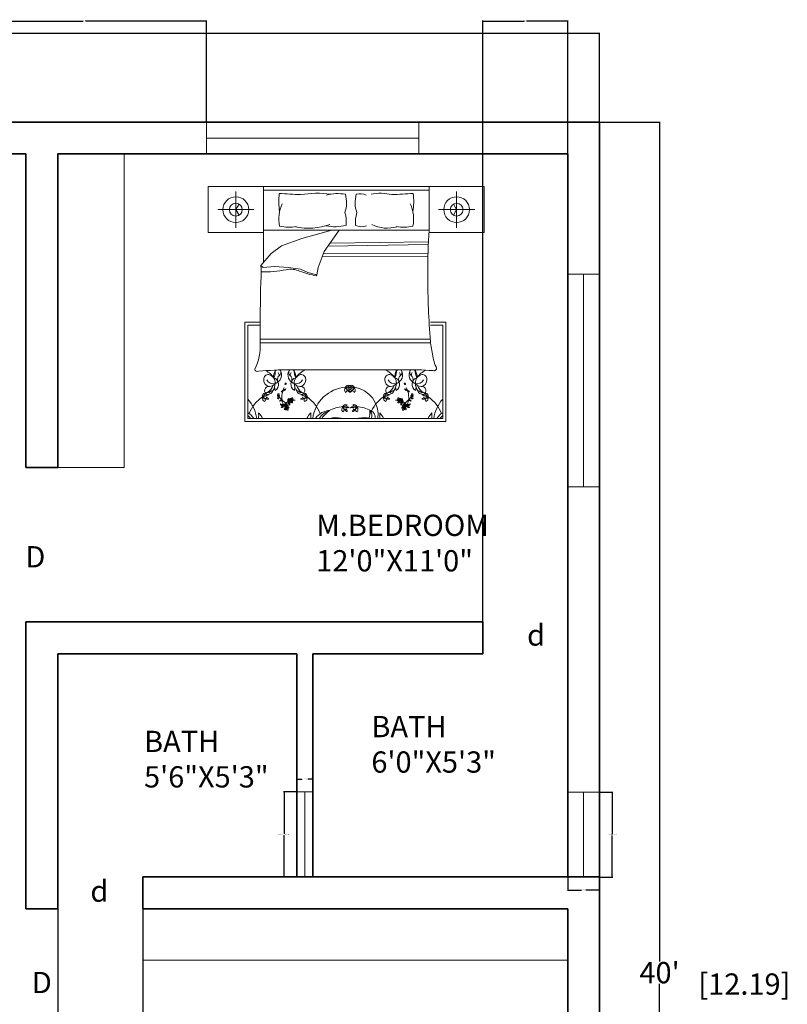
# Model space of a CAD drawing. Units: inches. Extents: x -43 to 1296, y -568 to 542.
# Tile 13 of 14: x 1020 to 1237, y -253 to 25. Entities that reach past the tile are written whole.
import ezdxf

# ---------------------------------------------------------------- set-up
doc = ezdxf.new("R2010")
doc.units = ezdxf.units.IN
doc.header["$MEASUREMENT"] = 0
for name, color, linetype, lineweight in [('A-ANNO-DIMS', 2, 'Continuous', 18), ('A-ANNO-TEXT', 7, 'Continuous', 18), ('A-AREA-IDEN', 7, 'Continuous', 18), ('A-FLOR-CASE', 9, 'Continuous', 18), ('A-FURN', 8, 'Continuous', 13), ('A-GLAZ', 6, 'Continuous', 18), ('A-WALL', 7, 'Continuous', 35)]:
    doc.layers.add(name, color=color, linetype=linetype, lineweight=lineweight)
doc.styles.get("Standard").update_dxf_attribs({"font": 'arial.ttf'})
doc.dimstyles.get("Standard").update_dxf_attribs({"dimtxt": 0.18, "dimasz": 0.18, "dimexe": 0.18, "dimexo": 0.0625, "dimgap": 0.09, "dimtad": 0, "dimtih": 1, "dimtoh": 1, "dimdec": 0, "dimzin": 0, "dimdsep": 46, "dimlunit": 3, "dimtxsty": 'Standard', "dimcen": 0.09, "dimadec": 0, "dimazin": 0, "dimtfac": 1, "dimtdec": 0, "dimtofl": 0, "dimtmove": 0, "dimatfit": 3, "dimfxl": 1, "dimtolj": 1, "dimtzin": 0, "dimarcsym": 0})

# ---------------------------------------------------------------- blocks, each defined once
blk = doc.blocks.new('*D3')
at = {"layer": 'A-ANNO-DIMS', "color": 0, "lineweight": -2, "transparency": 16777216}
for p, q in [((824.13, -3.7), (824.13, 21.38)), ((824.31, 21.2), (998.95, 21.2)), ((1183.95, 21.2), (1009.31, 21.2)), ((1184.13, -3.7), (1184.13, 21.38))]:
    blk.add_line(p, q, dxfattribs=at)
at = {"layer": 'A-ANNO-DIMS', "color": 0, "transparency": 16777216}
for points in [[(824.31, 21.23), (824.31, 21.17), (824.13, 21.2)], [(1183.95, 21.23), (1183.95, 21.17), (1184.13, 21.2)]]:
    blk.add_solid(points, dxfattribs=at)
at = {"layer": 'Defpoints', "color": 0, "transparency": 16777216}
for p in [(1184.13, 21.2), (824.13, -3.76), (1184.13, -3.76)]:
    blk.add_point(p, dxfattribs=at)
at = {"layer": 'A-ANNO-DIMS', "color": 0, "transparency": 16777216, "insert": (1004.13, 21.2), "char_height": 6, "attachment_point": 5}
blk.add_mtext("\\A1;30'", dxfattribs=at)
blk = doc.blocks.new('*D4')
at = {"layer": 'A-ANNO-DIMS', "color": 0, "lineweight": -2, "transparency": 16777216}
for p, q in [((1184.19, -3.76), (1201.25, -3.76)), ((1201.07, -3.94), (1201.07, -240.61)), ((1201.07, -483.58), (1201.07, -246.91)), ((1184.19, -483.76), (1201.25, -483.76))]:
    blk.add_line(p, q, dxfattribs=at)
at = {"layer": 'A-ANNO-DIMS', "color": 0, "transparency": 16777216}
for points in [[(1201.04, -3.94), (1201.1, -3.94), (1201.07, -3.76)], [(1201.04, -483.58), (1201.1, -483.58), (1201.07, -483.76)]]:
    blk.add_solid(points, dxfattribs=at)
at = {"layer": 'Defpoints', "color": 0, "transparency": 16777216}
for p in [(1184.13, -3.76), (1184.13, -483.76), (1201.07, -483.76)]:
    blk.add_point(p, dxfattribs=at)
at = {"layer": 'A-ANNO-DIMS', "color": 0, "transparency": 16777216, "insert": (1201.07, -243.76), "char_height": 6, "attachment_point": 5}
blk.add_mtext("\\A1;40'", dxfattribs=at)
blk = doc.blocks.new('BED-SUITE-78')
for p, q in [((0, 66.29), (77.95, 66.29)), ((7.79, 54.7), (7.79, 64.89)), ((15.59, 66.29), (15.59, 44.89)), ((62.36, 65.29), (15.59, 65.29)), ((70.15, 54.7), (70.15, 64.89)), ((12.89, 59.79), (2.7, 59.79)), ((65.06, 59.79), (75.25, 59.79)), ((15.59, 53.97), (62.36, 53.97)), ((26.42, 51.65), (34.92, 53.97)), ((37, 53.97), (32.73, 48.03)), ((20.73, 49.6), (26.42, 51.65)), ((62.15, 50.73), (34.4, 50.34)), ((14.89, 44.08), (17.73, 47.39)), ((17.73, 47.39), (20.73, 49.6)), ((32.73, 48.03), (31, 43.45)), ((62.08, 47.48), (32.48, 47.36)), ((62.12, 49.93), (33.82, 49.53)), ((62.08, 46.68), (32.17, 46.56)), ((15.52, 43.45), (14.89, 44.08)), ((18.68, 43.77), (15.52, 43.45)), ((22.63, 43.45), (18.68, 43.77)), ((26.1, 42.98), (22.63, 43.45)), ((28.15, 42.03), (26.1, 42.98)), ((30.68, 41.4), (28.15, 42.03)), ((31, 43.45), (30.68, 41.4)), ((10.29, 28.08), (14.7, 28.08)), ((10.29, 0), (10.29, 28.08)), ((62.79, 28.08), (67.12, 28.08)), ((67.12, 28.08), (67.12, 0)), ((14.7, 27.18), (11.19, 27.18)), ((11.19, 27.18), (11.19, 0.9)), ((66.21, 27.18), (62.78, 27.18)), ((66.21, 0.9), (66.21, 27.18)), ((62.71, 23.22), (14.69, 23.22)), ((62.79, 22.25), (14.69, 22.25)), ((54.8, 14.59), (23.15, 14.59)), ((18.87, 8.81), (18.7, 9.69)), ((24.32, 8.81), (24.49, 9.69)), ((53.08, 8.81), (52.91, 9.69)), ((58.53, 8.81), (58.7, 9.69)), ((67.12, 0), (10.29, 0)), ((11.19, 0.9), (66.21, 0.9))]:
    blk.add_line(p, q)
for points in [[(15.59, 53.3), (0, 53.3), (0, 66.29)], [(62.36, 66.29), (62.36, 53.3), (77.95, 53.3), (77.95, 66.29)], [(7.79, 59.79), (8.7, 61.37)], [(70.15, 59.79), (69.24, 61.37)], [(7.79, 59.79), (8.7, 58.22)], [(70.15, 59.79), (69.24, 58.22)]]:
    blk.add_lwpolyline(points)
for points in [[(20.07, 64.35, 0.074897), (20.16, 59.26, -0.472817)], [(38.61, 58.97, 0.14099), (38.76, 64.16, 0.235245)], [(41.94, 58.97, -0.14099), (41.78, 64.16, -0.235245)], [(57.88, 64.35, -0.074897), (57.79, 59.26, 0.472817)], [(14.73, 36.94, 0.001242), (14.69, 22.15, -0.127202), (13.13, 14.78)], [(62.69, 23.83, 0.056112), (63.26, 19.54, 0.095341), (64.35, 15.41)]]:
    blk.add_lwpolyline(points, format="xyb")
for centre, radius in [((7.79, 59.79), 3.64), ((7.79, 59.79), 1.82), ((70.15, 59.79), 3.64), ((70.15, 59.79), 1.82), ((23.38, 5.98), 0.199), ((54.03, 5.98), 0.199), ((22.08, 3.89), 0.199), ((55.33, 3.89), 0.199)]:
    blk.add_circle(centre, radius)
for centre, radius, start, end in [((63.03, 806.15), 743.04, 266.68521, 267.14978), ((30.75, 36.14), 28.27, 82.2196, 99.497), ((36.72, 50.43), 13.89, 81.5249, 103.96), ((42.85, 60.46), 3.86, 63.3437, 106.1026), ((48.63, 50.71), 13.7, 76.3427, 101.1841), ((14.92, 806.15), 743.04, 272.85022, 273.31479), ((30, 57.21), 10.05, 155.1316, 191.7583), ((47.95, 57.21), 10.05, 348.2417, 24.8684), ((29.42, 56.37), 9.55, 354.0129, 15.8293), ((51.13, 56.37), 9.55, 164.1707, 185.9871), ((28.35, 72.68), 18.12, 258.0397, 289.2615), ((50.59, 64.49), 9.92, 243.8761, 286.1746), ((22.85, 65.26), 10.45, 255.1039, 281.0369), ((35.68, 68.73), 13.75, 259.8617, 283.6238), ((43.37, 59.11), 4.13, 245.0183, 288.5407), ((55.1, 65.26), 10.45, 258.9631, 284.8961), ((202.09, 44.45), 140.06, 176.1, 180.9282), ((-56.58, 42.14), 71.5, 355.8294, 1.553), ((16.23, 71.68), 29.42, 267.4519, 281.3392), ((23.26, 36.62), 6.35, 66.2616, 101.3392), ((36.09, 70.85), 30.23, 250.1194, 259.3383), ((244.73, 39.35), 182.7, 179.1145, 184.8735), ((30.5, 41.34), 0.188, 268.8623, 19.7536), ((13.85, 14.83), 0.719, 183.98, 297.3412), ((22.22, -66.55), 81.14, 89.3433, 95.6887), ((13.54, 9.1), 5.9, 33.6671, 63.2997), ((21.45, 12.61), 3.01, 145.785, 184.7304), ((15.71, 14.01), 3.23, 328.8218, 9.1554), ((19.71, 13.73), 0.939, 120.0293, 142.325), ((18.21, 13.17), 2.48, 289.2822, 29.1751), ((19.31, 13.91), 1.17, 311.5653, 23.8354), ((19.71, 13.73), 0.939, 44.4517, 63.558), ((24.99, 13.17), 2.48, 150.8249, 250.7178), ((23.88, 13.91), 1.17, 156.1646, 228.4347), ((23.49, 13.73), 0.939, 113.229, 135.5483), ((23.49, 13.73), 0.939, 37.675, 66.7144), ((21.74, 12.61), 3.01, 355.2696, 34.215), ((27.49, 14.01), 3.23, 169.7133, 211.1782), ((29.65, 9.1), 5.9, 111.4941, 146.3329), ((47.75, 9.1), 5.9, 33.6671, 68.5059), ((55.66, 12.61), 3.01, 145.785, 184.7304), ((49.92, 14.01), 3.23, 328.8218, 10.2867), ((53.92, 13.73), 0.939, 113.2856, 142.325), ((52.42, 13.17), 2.48, 289.2822, 29.1751), ((53.92, 13.73), 0.939, 44.4517, 66.7144), ((53.52, 13.91), 1.17, 311.5653, 23.8354), ((57.18, -61.22), 75.85, 85.2402, 91.8035), ((59.2, 13.17), 2.48, 150.8249, 250.7178), ((58.09, 13.91), 1.17, 156.1646, 228.4347), ((57.7, 13.73), 0.939, 106.6343, 135.5483), ((57.7, 13.73), 0.939, 37.675, 72.5814), ((55.96, 12.61), 3.01, 355.2696, 34.215), ((61.7, 14.01), 3.23, 169.249, 211.1782), ((63.86, 9.1), 5.9, 113.6453, 146.3329), ((63.76, 15.02), 0.71, 246.5219, 33.8264), ((16.98, 11.93), 1.32, 84.4856, 181.0538), ((17.52, 11.74), 1.86, 174.9449, 262.8857), ((18.25, 12.45), 1.81, 201.5819, 291.4221), ((16.58, 10.96), 2.34, 355.2933, 76.921), ((17.91, 10.49), 1.94, 299.9085, 73.1337), ((19.13, 11.3), 0.484, 257.3041, 15.1471), ((21.14, 11.84), 1.6, 131.5653, 195.1471), ((17.83, 12.72), 2.24, 7.436, 29.9149), ((22.05, 11.84), 1.6, 344.8529, 48.4347), ((25.36, 12.72), 2.24, 150.0851, 172.564), ((25.29, 10.49), 1.94, 106.8663, 240.0915), ((24.06, 11.3), 0.484, 164.8529, 282.6959), ((26.62, 10.96), 2.34, 103.079, 184.7067), ((24.94, 12.45), 1.81, 248.5779, 338.4181), ((25.68, 11.74), 1.86, 277.1143, 5.0551), ((26.21, 11.93), 1.32, 358.9462, 95.5144), ((51.19, 11.93), 1.32, 84.4856, 181.0538), ((51.73, 11.74), 1.86, 174.9449, 262.8857), ((52.46, 12.45), 1.81, 201.5819, 291.4221), ((50.79, 10.96), 2.34, 355.2933, 76.921), ((52.12, 10.49), 1.94, 299.9085, 73.1337), ((53.34, 11.3), 0.484, 257.3041, 15.1471), ((55.35, 11.84), 1.6, 131.5653, 195.1471), ((52.04, 12.72), 2.24, 7.436, 29.9149), ((56.26, 11.84), 1.6, 344.8529, 48.4347), ((59.57, 12.72), 2.24, 150.0851, 172.564), ((59.5, 10.49), 1.94, 106.8663, 240.0915), ((58.27, 11.3), 0.484, 164.8529, 282.6959), ((60.83, 10.96), 2.34, 103.079, 184.7067), ((59.15, 12.45), 1.81, 248.5779, 338.4181), ((59.89, 11.74), 1.86, 277.1143, 5.0551), ((60.42, 11.93), 1.32, 358.9462, 95.5144), ((17.09, 8.74), 1.17, 80.264, 250.8688), ((14.77, 11.32), 3.68, 301.2614, 341.7045), ((16.81, 9.09), 1.46, 265.969, 344.3045), ((18.38, 7.15), 1.56, 96.1662, 141.5825), ((17.19, 12.16), 2.26, 272.3591, 324.0401), ((14.74, 11.02), 4.18, 326.2883, 356.5076), ((21.45, 12.61), 3.01, 212.7011, 216.3445), ((20.96, 8.24), 0.409, 101.3256, 154.4621), ((20.37, 9.63), 1.23, 280.2588, 300.656), ((20.65, 10.62), 2.2, 268.3264, 277.1302), ((27.22, 6.64), 6.46, 163.5842, 183.8277), ((20.1, 9.63), 1.25, 308.2101, 316.3071), ((20.87, 8.81), 0.374, 278.3432, 4.2869), ((20.67, 9.14), 0.653, 300.656, 332.6341), ((21.16, 8.7), 0.159, 55.7657, 157.4417), ((27.22, 6.64), 6.46, 153.0032, 159.8941), ((21.4, 8.85), 0.159, 84.3784, 186.0543), ((21.26, 9.49), 0.653, 269.1859, 301.164), ((21.45, 9.15), 0.374, 237.5332, 323.4768), ((21.08, 10.22), 1.25, 285.5129, 293.6099), ((20.96, 9.98), 1.23, 301.164, 321.5612), ((21.9, 8.81), 0.409, 87.3579, 140.4944), ((21.82, 10.57), 0.15, 102.7051, 280.4384), ((19.95, 10.2), 2.2, 324.6898, 333.4936), ((21.8, 10.66), 0.244, 280.4384, 100.4136), ((21.74, 12.61), 3.01, 323.6555, 327.2989), ((26, 12.16), 2.26, 215.9599, 267.6409), ((28.46, 11.02), 4.18, 183.4924, 213.7117), ((28.42, 11.32), 3.68, 198.2955, 238.7386), ((24.81, 7.15), 1.56, 38.4175, 83.8338), ((26.38, 9.09), 1.46, 195.6955, 274.031), ((26.1, 8.74), 1.17, 289.1312, 99.736), ((39.58, -0.47), 10.18, 94.4623, 172.255), ((39.62, 8.92), 1.13, 137.7873, 219.1145), ((38.34, 8.96), 0.85, 298.5391, 58.3627), ((39.6, 9.44), 0.844, 63.0274, 163.8037), ((38.74, 11.42), 1.74, 271.4585, 315.3727), ((39.45, 8.21), 1.61, 45.5411, 114.3101), ((40.92, 16.47), 7.12, 252.593, 267.2582), ((39.62, 9.65), 0.833, 177.7585, 283.852), ((41.22, 10.51), 2.57, 198.9159, 238.011), ((40.55, 8.21), 1.61, 65.6899, 134.4589), ((39.08, 16.47), 7.12, 272.7418, 287.407), ((39.79, 8.95), 0.11, 283.852, 219.9245), ((39.93, 8.44), 0.126, 238.011, 71.5592), ((39.95, 8.5), 0.0614, 71.5592, 188.0167), ((40.08, 8.44), 0.126, 108.4408, 301.989), ((40.4, 9.44), 0.844, 16.1963, 116.9726), ((41.26, 11.42), 1.74, 224.6273, 268.5415), ((40.06, 8.5), 0.0614, 351.9833, 108.4408), ((40.2, 8.99), 0.0664, 320.1909, 256.0209), ((38.78, 10.51), 2.57, 301.989, 341.0841), ((40.38, 9.65), 0.833, 256.148, 2.2415), ((41.66, 8.96), 0.85, 121.6373, 241.4609), ((40.38, 8.92), 1.13, 320.8855, 42.2127), ((40.09, 1.88), 7.88, 352.8636, 81.8197), ((51.3, 8.74), 1.17, 80.264, 250.8688), ((48.98, 11.32), 3.68, 301.2614, 341.7045), ((51.02, 9.09), 1.46, 265.969, 344.3045), ((52.59, 7.15), 1.56, 96.1662, 141.5825), ((51.4, 12.16), 2.26, 272.3591, 324.0401), ((48.95, 11.02), 4.18, 326.2883, 356.5076), ((55.66, 12.61), 3.01, 212.7011, 216.3445), ((55.6, 10.66), 0.244, 79.5864, 259.5616), ((56.45, 9.98), 1.23, 218.4388, 238.836), ((55.5, 8.81), 0.409, 39.5056, 92.6421), ((57.45, 10.2), 2.2, 206.5064, 215.3102), ((55.58, 10.57), 0.15, 259.5616, 77.2949), ((55.96, 9.15), 0.374, 216.5232, 302.4668), ((56.15, 9.49), 0.653, 238.836, 270.8141), ((56.32, 10.22), 1.25, 246.3901, 254.4871), ((50.18, 6.64), 6.46, 20.1059, 26.9968), ((56, 8.85), 0.159, 353.9457, 95.6216), ((56.25, 8.7), 0.159, 22.5583, 124.2343), ((56.53, 8.81), 0.374, 175.7131, 261.6568), ((56.74, 9.14), 0.653, 207.3659, 239.344), ((50.18, 6.64), 6.46, 356.1723, 16.4158), ((57.3, 9.63), 1.25, 223.6929, 231.7899), ((57.03, 9.63), 1.23, 239.344, 259.7412), ((56.75, 10.62), 2.2, 262.8698, 271.6736), ((56.44, 8.24), 0.409, 25.5379, 78.6744), ((55.96, 12.61), 3.01, 323.6555, 327.2989), ((60.21, 12.16), 2.26, 215.9599, 267.6409), ((62.67, 11.02), 4.18, 183.4924, 213.7117), ((62.63, 11.32), 3.68, 198.2955, 238.7386), ((60.59, 9.09), 1.46, 195.6955, 274.031), ((59.02, 7.15), 1.56, 38.4175, 83.8338), ((60.31, 8.74), 1.17, 289.1312, 99.736), ((3.61, -0.47), 10.18, 7.745, 41.8856), ((21.03, -1.47), 10.18, 124.3865, 158.5908), ((16.38, 6.69), 1.13, 167.7115, 249.0387), ((16.1, 7.13), 0.844, 92.9516, 193.728), ((14.37, 8.41), 1.74, 301.3827, 345.2969), ((16.59, 5.98), 1.61, 75.4653, 144.2343), ((13.74, 13.88), 7.12, 282.5173, 297.1824), ((15.25, 6.08), 0.85, 328.4633, 88.2869), ((16.97, 8.86), 2.57, 228.8402, 267.9352), ((16.02, 7.31), 0.833, 207.6827, 313.7762), ((16.85, 7.48), 0.717, 63.9755, 143.2681), ((16.52, 6.79), 0.11, 313.7762, 249.7183), ((16.87, 6.48), 0.0614, 101.4834, 217.9409), ((16.89, 6.42), 0.126, 267.9352, 101.4834), ((19.8, 7.47), 0.331, 101.5637, 142.6358), ((19.53, 7.16), 0.199, 273.2768, 86.7232), ((19.8, 6.79), 0.328, 217.7621, 259.0403), ((19.76, 7.35), 0.19, 91.1081, 181.8675), ((20.15, 7.23), 0.603, 203.4276, 227.6104), ((19.96, 6.97), 0.41, 80.3487, 133.6538), ((19.89, 7.31), 0.325, 229.7889, 317.6792), ((19.54, 7.73), 0.477, 288.7263, 352.5032), ((19.52, 6.62), 0.461, 355.053, 68.3618), ((19.88, 6.54), 0.65, 83.0852, 105.7171), ((19.86, 7.7), 0.153, 345.2356, 144.9248), ((19.83, 6.59), 0.152, 232.4737, 355.053), ((15.38, 1.15), 7.4, 43.1541, 52.0459), ((20, 7.2), 0.171, 317.6792, 80.3487), ((20.5, 5.62), 0.409, 101.3256, 154.4621), ((19.91, 7.01), 1.23, 280.2588, 300.656), ((20.19, 8), 2.2, 268.3264, 277.1302), ((19.64, 7.01), 1.25, 308.2101, 316.3071), ((20.41, 6.18), 0.374, 278.3432, 4.2869), ((20.2, 6.51), 0.653, 300.656, 332.6341), ((20.69, 6.08), 0.159, 55.7657, 157.4417), ((24.01, 6.48), 3.24, 184.756, 209.2041), ((28.67, 13.37), 10.65, 222.2412, 232.1744), ((21.86, 6.28), 0.905, 304.5369, 16.3699), ((22.34, 6.07), 0.55, 272.8499, 356.1226), ((21.95, 5.86), 0.533, 321.7607, 7.9252), ((23.11, 6.02), 0.64, 127.3105, 187.9252), ((22.23, 6.09), 0.657, 355.0106, 41.658), ((22.96, 5.61), 0.197, 148.0499, 225.6268), ((24.34, 2.18), 3.88, 113.0501, 113.8477), ((23.32, 5.38), 0.626, 104.7558, 148.0499), ((22.97, 5.83), 0.392, 247.4086, 351.4386), ((23.16, 6.26), 0.271, 126.1046, 271.4281), ((23.13, 6.33), 0.194, 353.7526, 131.7054), ((23.08, 5.81), 0.131, 262.906, 7.132), ((22.94, 6.1), 0.273, 0.0645, 61.1507), ((23.01, 6.33), 0.312, 311.8413, 355.7877), ((23.65, 6.29), 0.331, 101.5637, 176.365), ((23.65, 5.61), 0.328, 151.2196, 259.0403), ((23.61, 6.17), 0.19, 91.1081, 181.8675), ((24, 6.05), 0.603, 203.4276, 227.6104), ((23.81, 5.79), 0.41, 80.3487, 133.6538), ((23.74, 6.13), 0.325, 229.7889, 317.6792), ((23.38, 6.55), 0.477, 288.7263, 352.5032), ((23.37, 5.44), 0.461, 355.053, 68.3618), ((23.73, 5.36), 0.65, 83.0852, 105.7171), ((23.71, 6.53), 0.153, 345.2356, 144.9248), ((23.85, 6.02), 0.171, 317.6792, 80.3487), ((24.34, 2.18), 3.88, 87.1071, 94.7585), ((26.34, 7.48), 0.717, 36.7319, 116.0245), ((26.31, 6.42), 0.126, 78.5166, 272.0648), ((26.61, 5.98), 1.61, 35.7657, 104.5347), ((29.46, 13.88), 7.12, 242.8176, 257.4827), ((26.22, 8.86), 2.57, 272.0648, 311.1598), ((26.32, 6.48), 0.0614, 322.0591, 78.5166), ((27.18, 7.31), 0.833, 226.2238, 332.3173), ((26.69, 6.83), 0.0664, 290.2667, 226.2271), ((27.94, 6.08), 0.85, 91.7131, 211.5367), ((27.09, 7.13), 0.844, 346.272, 87.0484), ((28.82, 8.41), 1.74, 194.7031, 238.6173), ((26.81, 6.69), 1.13, 290.9613, 12.2885), ((22.17, -1.47), 10.18, 21.4092, 55.6135), ((55.24, -1.47), 10.18, 124.3865, 158.5908), ((50.59, 6.69), 1.13, 167.7115, 249.0387), ((50.31, 7.13), 0.844, 92.9516, 193.728), ((48.58, 8.41), 1.74, 301.3827, 345.2969), ((50.8, 5.98), 1.61, 75.4653, 144.2343), ((47.95, 13.88), 7.12, 282.5173, 297.1824), ((50.23, 7.31), 0.833, 207.6827, 313.7762), ((51.18, 8.86), 2.57, 228.8402, 267.9352), ((49.46, 6.08), 0.85, 328.4633, 88.2869), ((51.06, 7.48), 0.717, 63.9755, 143.2681), ((50.73, 6.79), 0.11, 313.7762, 249.7183), ((51.08, 6.48), 0.0614, 101.4834, 217.9409), ((51.1, 6.42), 0.126, 267.9352, 101.4834), ((53.06, 2.18), 3.88, 85.2415, 92.8929), ((53.55, 6.02), 0.171, 99.6513, 222.3208), ((53.67, 6.13), 0.325, 222.3208, 310.2111), ((53.59, 5.79), 0.41, 46.3462, 99.6513), ((53.69, 6.53), 0.153, 35.0752, 194.7644), ((54.02, 6.55), 0.477, 187.4968, 251.2737), ((54.03, 5.44), 0.461, 111.6382, 184.947), ((53.67, 5.36), 0.65, 74.2829, 96.9148), ((53.8, 6.17), 0.19, 358.1325, 88.8919), ((53.4, 6.05), 0.603, 312.3896, 336.5724), ((53.75, 6.29), 0.331, 3.635, 78.4363), ((53.76, 5.61), 0.328, 280.9597, 28.7804), ((54.43, 5.83), 0.392, 188.5614, 292.5914), ((54.28, 6.33), 0.194, 48.2946, 186.2474), ((54.39, 6.33), 0.312, 184.2123, 228.1587), ((54.46, 6.1), 0.273, 118.8493, 179.9355), ((54.32, 5.81), 0.131, 172.868, 277.094), ((54.25, 6.26), 0.271, 268.5719, 53.8954), ((54.08, 5.38), 0.626, 31.9501, 75.2442), ((55.17, 6.09), 0.657, 138.342, 184.9894), ((55.06, 6.07), 0.55, 183.8774, 267.1501), ((53.06, 2.18), 3.88, 66.1523, 66.9499), ((54.44, 5.61), 0.197, 314.3732, 31.9501), ((55.55, 6.28), 0.905, 163.6301, 235.4631), ((54.29, 6.02), 0.64, 352.0748, 52.6895), ((55.45, 5.86), 0.533, 172.0748, 218.2393), ((48.74, 13.37), 10.65, 307.8256, 317.7588), ((53.4, 6.48), 3.24, 330.7959, 355.244), ((62.02, 1.15), 7.4, 127.9541, 136.8459), ((56.71, 6.08), 0.159, 22.5583, 124.2343), ((57, 6.18), 0.374, 175.7131, 261.6568), ((57.2, 6.51), 0.653, 207.3659, 239.344), ((57.76, 7.01), 1.25, 223.6929, 231.7899), ((57.5, 7.01), 1.23, 239.344, 259.7412), ((57.21, 8), 2.2, 262.8698, 271.6736), ((56.91, 5.62), 0.409, 25.5379, 78.6744), ((57.4, 7.2), 0.171, 99.6513, 222.3208), ((57.52, 7.31), 0.325, 222.3208, 310.2111), ((57.44, 6.97), 0.41, 46.3462, 99.6513), ((57.54, 7.7), 0.153, 35.0752, 194.7644), ((57.87, 7.73), 0.477, 187.4968, 251.2737), ((57.88, 6.62), 0.461, 111.6382, 184.947), ((57.57, 6.59), 0.152, 184.947, 307.5263), ((57.52, 6.54), 0.65, 74.2829, 96.9148), ((57.64, 7.35), 0.19, 358.1325, 88.8919), ((57.25, 7.23), 0.603, 312.3896, 336.5724), ((57.6, 7.47), 0.331, 37.3642, 78.4363), ((57.61, 6.79), 0.328, 280.9597, 322.2379), ((57.88, 7.16), 0.199, 93.2768, 266.7232), ((60.55, 7.48), 0.717, 36.7319, 116.0245), ((60.52, 6.42), 0.126, 78.5166, 272.0648), ((60.82, 5.98), 1.61, 35.7657, 104.5347), ((63.67, 13.88), 7.12, 242.8176, 257.4827), ((60.43, 8.86), 2.57, 272.0648, 311.1598), ((60.53, 6.48), 0.0614, 322.0591, 78.5166), ((61.39, 7.31), 0.833, 226.2238, 332.3173), ((60.9, 6.83), 0.0664, 290.2667, 226.2271), ((62.15, 6.08), 0.85, 91.7131, 211.5367), ((63.03, 8.41), 1.74, 194.7031, 238.6173), ((61.3, 7.13), 0.844, 346.272, 87.0484), ((61.02, 6.69), 1.13, 290.9613, 12.2885), ((56.38, -1.47), 10.18, 21.4092, 55.6135), ((73.79, -0.47), 10.18, 138.1144, 172.255), ((20.63, 4.9), 0.222, 146.8636, 236.9021), ((23.76, 9.79), 5.8, 235.1882, 238.8844), ((21.01, 5.22), 0.6, 199.4799, 267.6828), ((20.95, 5), 0.517, 212.8155, 277.3992), ((20.65, 4.65), 0.6, 266.9701, 338.2913), ((17.48, 8.93), 5.8, 302.6784, 306.3746), ((20.8, 4.18), 0.222, 214.3538, 304.3923), ((20.88, 5.02), 0.229, 238.8844, 314.2646), ((20.83, 4.5), 0.517, 280.3057, 17.1958), ((20.79, 4.45), 0.229, 306.3746, 21.7548), ((21.16, 4.6), 0.173, 19.3605, 201.7548), ((21.16, 4.73), 0.173, 311.8703, 134.2646), ((24.42, 3.15), 3.46, 153.7819, 158.2913), ((21.66, 5.51), 0.905, 247.2305, 319.0635), ((21.37, 5.21), 0.533, 264.4544, 310.6188), ((24.01, 6.48), 3.24, 214.0033, 222.4917), ((21.76, 5), 0.55, 218.3208, 298.8162), ((24.34, 2.18), 3.88, 120.544, 139.818), ((21.66, 3.52), 0.197, 148.0499, 225.6268), ((22.02, 3.29), 0.626, 104.7558, 148.0499), ((21.67, 3.74), 0.392, 247.4086, 351.4386), ((21.86, 4.17), 0.271, 126.1046, 271.4281), ((21.83, 4.24), 0.194, 353.7526, 131.7054), ((22.13, 4.32), 0.64, 70.0041, 130.6188), ((21.78, 3.72), 0.131, 262.906, 7.132), ((21.65, 4.01), 0.273, 0.0645, 61.1507), ((21.71, 4.24), 0.312, 311.8413, 355.7877), ((21.71, 5.1), 0.657, 297.7043, 344.3516), ((22.35, 4.2), 0.331, 101.5637, 176.365), ((22.35, 3.52), 0.328, 151.2196, 259.0403), ((22.31, 4.08), 0.19, 91.1081, 181.8675), ((22.7, 3.96), 0.603, 203.4276, 227.6104), ((22.51, 3.7), 0.41, 80.3487, 133.6538), ((22.44, 4.04), 0.325, 229.7889, 317.6792), ((22.09, 4.46), 0.477, 288.7263, 352.5032), ((22.07, 3.35), 0.461, 355.053, 68.3618), ((22.43, 3.27), 0.65, 83.0852, 105.7171), ((22.41, 4.43), 0.153, 345.2356, 144.9248), ((22.38, 3.32), 0.152, 232.4737, 355.053), ((22.06, 5.1), 0.533, 8.7227, 54.8872), ((22.09, 4.67), 0.905, 0.278, 72.111), ((22.5, 5), 0.55, 20.5253, 88.5375), ((22.55, 3.93), 0.171, 317.6792, 80.3487), ((23.22, 5.27), 0.64, 188.7227, 249.3375), ((22.4, 4.95), 0.657, 334.9899, 21.6373), ((23.68, 5.41), 0.152, 232.4737, 355.053), ((34.47, -1.83), 4.96, 91.272, 146.5383), ((36.26, -2.76), 6.18, 107.8504, 143.6964), ((39.51, -4.49), 9.19, 124.0123, 144.053), ((38.8, -5.92), 10.18, 94.4623, 117.4146), ((38.84, 3.47), 1.13, 137.7873, 219.1145), ((37.56, 3.5), 0.85, 298.5391, 58.3627), ((38.82, 3.99), 0.844, 63.0274, 163.8037), ((37.96, 5.97), 1.74, 271.4585, 315.3727), ((38.67, 2.76), 1.61, 45.5411, 114.3101), ((40.44, 5.06), 2.57, 198.9159, 238.011), ((40.14, 11.02), 7.12, 252.593, 267.2582), ((38.84, 4.2), 0.833, 177.7585, 283.852), ((39.01, 3.49), 0.11, 283.852, 219.9245), ((39.15, 2.99), 0.126, 238.011, 71.5592), ((39.17, 3.05), 0.0614, 71.5592, 188.0167), ((41.33, 2.76), 1.61, 65.6899, 134.4589), ((39.86, 11.02), 7.12, 272.7418, 287.407), ((40.86, 2.99), 0.126, 108.4408, 301.989), ((41.18, 3.99), 0.844, 16.1963, 116.9726), ((42.04, 5.97), 1.74, 224.6273, 268.5415), ((40.83, 3.05), 0.0614, 351.9833, 108.4408), ((40.98, 3.54), 0.0664, 320.1909, 256.0209), ((39.56, 5.06), 2.57, 301.989, 341.0841), ((41.16, 4.2), 0.833, 256.148, 2.2415), ((42.44, 3.5), 0.85, 121.6373, 241.4609), ((41.16, 3.47), 1.13, 320.8855, 42.2127), ((41.2, -5.92), 10.18, 62.5854, 85.5377), ((41.11, 2.6), 4.56, 338.117, 6.6195), ((45.29, 1.33), 1.83, 346.3898, 79.0739), ((43.92, 1.58), 2.31, 342.8609, 41.9049), ((53.73, 5.41), 0.152, 184.947, 307.5263), ((55, 4.95), 0.657, 158.3627, 205.0101), ((54.91, 5), 0.55, 91.4625, 159.4747), ((55.31, 4.67), 0.905, 107.889, 179.722), ((54.18, 5.27), 0.64, 290.6625, 351.2773), ((54.85, 3.93), 0.171, 99.6513, 222.3208), ((54.97, 4.04), 0.325, 222.3208, 310.2111), ((55.34, 5.1), 0.533, 125.1128, 171.2773), ((54.89, 3.7), 0.41, 46.3462, 99.6513), ((54.99, 4.43), 0.153, 35.0752, 194.7644), ((55.32, 4.46), 0.477, 187.4968, 251.2737), ((55.33, 3.35), 0.461, 111.6382, 184.947), ((55.03, 3.32), 0.152, 184.947, 307.5263), ((54.97, 3.27), 0.65, 74.2829, 96.9148), ((53.06, 2.18), 3.88, 40.182, 59.456), ((55.27, 4.32), 0.64, 49.3812, 109.9959), ((55.74, 5.51), 0.905, 220.9365, 292.7695), ((55.69, 5.1), 0.657, 195.6484, 242.2957), ((55.09, 4.08), 0.19, 358.1325, 88.8919), ((54.7, 3.96), 0.603, 312.3896, 336.5724), ((55.05, 4.2), 0.331, 3.635, 78.4363), ((55.06, 3.52), 0.328, 280.9597, 28.7804), ((55.73, 3.74), 0.392, 188.5614, 292.5914), ((55.65, 5), 0.55, 241.1838, 321.6792), ((55.58, 4.24), 0.194, 48.2946, 186.2474), ((55.69, 4.24), 0.312, 184.2123, 228.1587), ((55.76, 4.01), 0.273, 118.8493, 179.9355), ((55.62, 3.72), 0.131, 172.868, 277.094), ((55.55, 4.17), 0.271, 268.5719, 53.8954), ((55.38, 3.29), 0.626, 31.9501, 75.2442), ((56.04, 5.21), 0.533, 229.3812, 275.5456), ((53.4, 6.48), 3.24, 317.5083, 325.9967), ((55.74, 3.52), 0.197, 314.3732, 31.9501), ((56.57, 4.5), 0.517, 162.8042, 259.6943), ((56.24, 4.73), 0.173, 45.7354, 228.1297), ((56.24, 4.6), 0.173, 338.2452, 160.6395), ((52.99, 3.15), 3.46, 21.7087, 26.2181), ((56.76, 4.65), 0.6, 201.7087, 273.0299), ((56.52, 5.02), 0.229, 225.7354, 301.1156), ((56.46, 5), 0.517, 262.6008, 327.1845), ((56.62, 4.45), 0.229, 158.2452, 233.6254), ((56.39, 5.22), 0.6, 272.3172, 340.5201), ((59.92, 8.93), 5.8, 233.6254, 237.3216), ((56.61, 4.18), 0.222, 235.6077, 325.6462), ((53.65, 9.79), 5.8, 301.1156, 304.8118), ((56.77, 4.9), 0.222, 303.0979, 33.1364), ((8.72, -1.83), 4.96, 33.4617, 60.1116), ((6.94, -2.76), 6.18, 36.3036, 46.4814), ((11.5, -0.68), 4.14, 22.5547, 48.9546), ((0.16, 1.54), 14.08, 357.4081, 3.6519), ((31.7, -0.68), 4.14, 131.0454, 157.4453), ((43.03, 1.54), 14.08, 176.3481, 182.5919), ((35.95, -4.45), 5.6, 73.5431, 107.0202), ((38.17, -7.33), 8.28, 94.3787, 95.6357), ((42.53, -13), 14.79, 109.7217, 109.9028), ((44.05, -4.45), 5.6, 72.9798, 106.4569), ((41.83, -7.33), 8.28, 84.3643, 85.6213), ((37.47, -13), 14.79, 70.0972, 70.2783), ((34.37, 1.54), 14.08, 357.4081, 3.6519), ((45.71, -0.68), 4.14, 22.5547, 48.9546), ((65.91, -0.68), 4.14, 131.0454, 157.4453), ((77.24, 1.54), 14.08, 176.3481, 182.5919), ((68.68, -1.83), 4.96, 119.8884, 146.5383), ((70.47, -2.76), 6.18, 133.5186, 143.6964)]:
    blk.add_arc(centre, radius, start, end)
blk = doc.blocks.new('WIN-60x9')
for p, q in [((0, 60), (0, 0)), ((9, 60), (0, 60)), ((4.5, 60), (4.5, 0)), ((9, 0), (9, 60)), ((0, 0), (9, 0))]:
    blk.add_line(p, q)
blk = doc.blocks.new('VENT-24x9')
for p, q in [((0, 0), (0, 24)), ((0, 24), (9, 24)), ((4.5, 24), (4.5, 0)), ((9, 24), (9, 0)), ((9, 0), (0, 0))]:
    blk.add_line(p, q)
blk = doc.blocks.new('VENT-24x4-5')
for p, q in [((4.5, 24), (0, 24)), ((0, 24), (0, 0)), ((2.25, 0), (2.25, 24)), ((4.5, 0), (4.5, 24)), ((0, 0), (4.5, 0))]:
    blk.add_line(p, q)
blk = doc.blocks.new('*D34')
at = {"layer": 'A-ANNO-DIMS', "color": 0, "lineweight": -2, "transparency": 16777216}
for p, q in [((1184.19, -192.86), (1187.91, -192.86)), ((1187.73, -193.04), (1187.73, -204.68)), ((1187.73, -216.68), (1187.73, -205.04)), ((1184.19, -216.86), (1187.91, -216.86))]:
    blk.add_line(p, q, dxfattribs=at)
at = {"layer": 'A-ANNO-DIMS', "color": 0, "transparency": 16777216}
for points in [[(1187.7, -193.04), (1187.76, -193.04), (1187.73, -192.86)], [(1187.7, -216.68), (1187.76, -216.68), (1187.73, -216.86)]]:
    blk.add_solid(points, dxfattribs=at)
at = {"layer": 'Defpoints', "color": 0, "transparency": 16777216}
for p in [(1184.13, -192.86), (1184.13, -216.86), (1187.73, -216.86)]:
    blk.add_point(p, dxfattribs=at)
at = {"layer": 'A-ANNO-DIMS', "color": 0, "transparency": 16777216, "insert": (1187.73, -204.86), "char_height": 0.18, "attachment_point": 5}
blk.add_mtext('\\A1;WALL VENT 2\'-0" TYP.', dxfattribs=at)
blk = doc.blocks.new('*D35')
at = {"layer": 'A-ANNO-DIMS', "color": 0, "lineweight": -2, "transparency": 16777216}
for p, q in [((1175.13, -216.92), (1175.13, -220.64)), ((1184.13, -216.92), (1184.13, -220.64)), ((1175.31, -220.46), (1178.99, -220.46)), ((1183.95, -220.46), (1180.27, -220.46))]:
    blk.add_line(p, q, dxfattribs=at)
at = {"layer": 'A-ANNO-DIMS', "color": 0, "transparency": 16777216}
for points in [[(1175.31, -220.43), (1175.31, -220.49), (1175.13, -220.46)], [(1183.95, -220.43), (1183.95, -220.49), (1184.13, -220.46)]]:
    blk.add_solid(points, dxfattribs=at)
at = {"layer": 'Defpoints', "color": 0, "transparency": 16777216}
for p in [(1175.13, -216.86), (1184.13, -216.86), (1175.13, -220.46)]:
    blk.add_point(p, dxfattribs=at)
at = {"layer": 'A-ANNO-DIMS', "color": 0, "transparency": 16777216, "insert": (1179.63, -220.46), "char_height": 0.18, "attachment_point": 5}
blk.add_mtext('\\A1;0\'-9" TYP.', dxfattribs=at)
blk = doc.blocks.new('*D36')
at = {"layer": 'A-ANNO-DIMS', "color": 0, "lineweight": -2, "transparency": 16777216}
for p, q in [((1098.57, -192.76), (1094.85, -192.76)), ((1095.03, -192.94), (1095.03, -204.58)), ((1095.03, -216.58), (1095.03, -204.94)), ((1098.57, -216.76), (1094.85, -216.76))]:
    blk.add_line(p, q, dxfattribs=at)
at = {"layer": 'A-ANNO-DIMS', "color": 0, "transparency": 16777216}
for points in [[(1095, -192.94), (1095.06, -192.94), (1095.03, -192.76)], [(1095, -216.58), (1095.06, -216.58), (1095.03, -216.76)]]:
    blk.add_solid(points, dxfattribs=at)
at = {"layer": 'Defpoints', "color": 0, "transparency": 16777216}
for p in [(1098.63, -192.76), (1095.03, -216.76), (1098.63, -216.76)]:
    blk.add_point(p, dxfattribs=at)
at = {"layer": 'A-ANNO-DIMS', "color": 0, "transparency": 16777216, "insert": (1095.03, -204.76), "char_height": 0.18, "attachment_point": 5}
blk.add_mtext('\\A1;PARTITION VENT 2\'-0" TYP.', dxfattribs=at)
blk = doc.blocks.new('*D37')
at = {"layer": 'A-ANNO-DIMS', "color": 0, "lineweight": -2, "transparency": 16777216}
for p, q in [((1098.63, -192.7), (1098.63, -188.98)), ((1098.81, -189.16), (1100.03, -189.16)), ((1102.95, -189.16), (1101.73, -189.16)), ((1103.13, -192.7), (1103.13, -188.98))]:
    blk.add_line(p, q, dxfattribs=at)
at = {"layer": 'A-ANNO-DIMS', "color": 0, "transparency": 16777216}
for points in [[(1098.81, -189.13), (1098.81, -189.19), (1098.63, -189.16)], [(1102.95, -189.13), (1102.95, -189.19), (1103.13, -189.16)]]:
    blk.add_solid(points, dxfattribs=at)
at = {"layer": 'Defpoints', "color": 0, "transparency": 16777216}
for p in [(1098.63, -189.16), (1098.63, -192.76), (1103.13, -192.76)]:
    blk.add_point(p, dxfattribs=at)
at = {"layer": 'A-ANNO-DIMS', "color": 0, "transparency": 16777216, "insert": (1100.88, -189.16), "char_height": 0.18, "attachment_point": 5}
blk.add_mtext('\\A1;0\'-4 1/2" TYP.', dxfattribs=at)
blk = doc.blocks.new('*D82')
at = {"layer": 'A-ANNO-DIMS', "color": 0, "lineweight": -2, "transparency": 16777216}
for p, q in [((1004.13, -3.7), (1004.13, 24.92)), ((1004.31, 24.74), (1038.3, 24.74)), ((1072.95, 24.74), (1038.96, 24.74)), ((1073.13, -3.7), (1073.13, 24.92))]:
    blk.add_line(p, q, dxfattribs=at)
at = {"layer": 'A-ANNO-DIMS', "color": 0, "transparency": 16777216}
for points in [[(1004.31, 24.77), (1004.31, 24.71), (1004.13, 24.74)], [(1072.95, 24.77), (1072.95, 24.71), (1073.13, 24.74)]]:
    blk.add_solid(points, dxfattribs=at)
at = {"layer": 'Defpoints', "color": 0, "transparency": 16777216}
for p in [(1073.13, 24.74), (1004.13, -3.76), (1073.13, -3.76)]:
    blk.add_point(p, dxfattribs=at)
at = {"layer": 'A-ANNO-DIMS', "color": 0, "transparency": 16777216, "insert": (1038.63, 24.74), "char_height": 0.18, "attachment_point": 5}
blk.add_mtext('\\A1;5\'-9"', dxfattribs=at)
blk = doc.blocks.new('*D83')
at = {"layer": 'A-ANNO-DIMS', "color": 0, "lineweight": -2, "transparency": 16777216}
for p, q in [((1031.13, -225.82), (1031.13, -532.44)), ((1055.13, -225.82), (1055.13, -532.44)), ((1031.31, -532.26), (1042.8, -532.26)), ((1054.95, -532.26), (1043.46, -532.26))]:
    blk.add_line(p, q, dxfattribs=at)
at = {"layer": 'A-ANNO-DIMS', "color": 0, "transparency": 16777216}
for points in [[(1031.31, -532.23), (1031.31, -532.29), (1031.13, -532.26)], [(1054.95, -532.23), (1054.95, -532.29), (1055.13, -532.26)]]:
    blk.add_solid(points, dxfattribs=at)
at = {"layer": 'Defpoints', "color": 0, "transparency": 16777216}
for p in [(1031.13, -225.76), (1055.13, -225.76), (1055.13, -532.26)]:
    blk.add_point(p, dxfattribs=at)
at = {"layer": 'A-ANNO-DIMS', "color": 0, "transparency": 16777216, "insert": (1043.13, -532.26), "char_height": 0.18, "attachment_point": 5}
blk.add_mtext('\\A1;2\'-0"', dxfattribs=at)
blk = doc.blocks.new('*D84')
at = {"layer": 'A-ANNO-DIMS', "color": 0, "lineweight": -2, "transparency": 16777216}
for p, q in [((1151.13, -153.7), (1151.13, 24.92)), ((1151.31, 24.74), (1162.8, 24.74)), ((1174.95, 24.74), (1163.46, 24.74)), ((1175.13, -192.8), (1175.13, 24.92))]:
    blk.add_line(p, q, dxfattribs=at)
at = {"layer": 'A-ANNO-DIMS', "color": 0, "transparency": 16777216}
for points in [[(1151.31, 24.77), (1151.31, 24.71), (1151.13, 24.74)], [(1174.95, 24.77), (1174.95, 24.71), (1175.13, 24.74)]]:
    blk.add_solid(points, dxfattribs=at)
at = {"layer": 'Defpoints', "color": 0, "transparency": 16777216}
for p in [(1175.13, 24.74), (1151.13, -153.76), (1175.13, -192.86)]:
    blk.add_point(p, dxfattribs=at)
at = {"layer": 'A-ANNO-DIMS', "color": 0, "transparency": 16777216, "insert": (1163.13, 24.74), "char_height": 0.18, "attachment_point": 5}
blk.add_mtext('\\A1;2\'-0"', dxfattribs=at)

msp = doc.modelspace()

# ---------------------------------------------------------------- linework, layer by layer
at = {"layer": 'A-FLOR-CASE'}
for p, q in [((1049.84, -101.26), (1049.84, -12.76)), ((1031.13, -101.26), (1049.84, -101.26)), ((1055.13, -225.76), (1055.13, -240.24)), ((1055.13, -240.24), (1175.13, -240.24))]:
    msp.add_line(p, q, dxfattribs=at)
at = {"layer": 'A-WALL'}
for p, q in [((824.13, -3.76), (1184.13, -3.76)), ((1184.13, -3.76), (1184.13, -483.76)), ((962.13, -12.76), (1022.13, -12.76)), ((1022.13, -12.76), (1022.13, -101.26)), ((1031.13, -12.76), (1031.13, -101.26)), ((1031.13, -12.76), (1175.13, -12.76)), ((1175.13, -12.76), (1175.13, -216.76)), ((1022.13, -101.26), (1031.13, -101.26)), ((1022.13, -144.76), (1022.13, -225.76)), ((1022.13, -144.76), (1151.13, -144.76)), ((1151.13, -153.76), (1151.13, -144.76)), ((1031.13, -153.76), (1031.13, -225.76)), ((1031.13, -153.76), (1098.63, -153.76)), ((1098.63, -153.76), (1098.63, -216.76)), ((1103.13, -153.76), (1103.13, -216.76)), ((1103.13, -153.76), (1151.13, -153.76)), ((1055.13, -216.76), (1098.63, -216.76)), ((1055.13, -216.76), (1055.13, -225.76)), ((1098.63, -216.76), (1103.13, -216.76)), ((1103.13, -216.76), (1184.13, -216.76)), ((1022.13, -225.76), (1031.13, -225.76)), ((1055.13, -225.76), (1175.13, -225.76)), ((1175.13, -225.76), (1175.13, -345.76))]:
    msp.add_line(p, q, dxfattribs=at)

# ---------------------------------------------------------------- block references
at = {"layer": 'A-FURN'}
msp.add_blockref('BED-SUITE-78', (1073.62, -88.26), dxfattribs=at)
at = {"layer": 'A-GLAZ'}
for name, p, rotation in [('WIN-60x9', (1073.13, -3.76), 270.0000000000002), ('VENT-24x4-5', (1103.13, -192.76), 180), ('VENT-24x9', (1184.13, -192.86), 180)]:
    msp.add_blockref(name, p, dxfattribs=dict(at, rotation=rotation))
msp.add_blockref('WIN-60x9', (1175.13, -106.63), dxfattribs=at)

# ---------------------------------------------------------------- texts
at = {"layer": 'A-ANNO-DIMS', "insert": (1212.04, -243.98), "char_height": 6, "attachment_point": 1}
msp.add_mtext('[12.19]', dxfattribs=at)
at = {"layer": 'A-ANNO-TEXT', "char_height": 6, "attachment_point": 1}
for s, insert in [('D', (1021.98, -123.41)), ('d', (1040.32, -217.76)), ('D', (1023.81, -243.54))]:
    msp.add_mtext(s, dxfattribs=dict(at, insert=insert))
at = {"layer": 'A-ANNO-TEXT', "insert": (1163.66, -145.5), "char_height": 6, "attachment_point": 1}
msp.add_mtext_dynamic_manual_height_columns('d', width=0.3471, gutter_width=1, heights=[0], dxfattribs=at)
at = {"layer": 'A-AREA-IDEN', "char_height": 6, "attachment_point": 1}
for s, insert in [('M.BEDROOM\\P12\'0"X11\'0"', (1104.12, -114.54)), ('BATH\\P6\'0"X5\'3"', (1119.69, -171.33)), ('BATH\\P5\'6"X5\'3"', (1055.49, -175.51))]:
    msp.add_mtext(s, dxfattribs=dict(at, insert=insert))

# ---------------------------------------------------------------- dimensions: what is measured, and where the dimension line sits
at = {"layer": 'A-ANNO-DIMS'}
for base, p1, p2, override, picture, middle in [((1184.13, 21.2), (824.13, -3.76), (1184.13, -3.76), {"dimtxt": 6, "dimclrd": 0, "dimclre": 0, "dimclrt": 0}, '*D3', (1004.13, 21.2)), ((1073.13, 24.74), (1004.13, -3.76), (1073.13, -3.76), {"dimdec": 1, "dimlfac": 1, "dimrnd": 0, "dimzin": 1, "dimdsep": 46, "dimlunit": 4, "dimfrac": 2}, '*D82', (1038.63, 24.74)), ((1175.13, 24.74), (1151.13, -153.76), (1175.13, -192.86), {"dimdec": 1, "dimlfac": 1, "dimrnd": 0, "dimzin": 1, "dimdsep": 46, "dimlunit": 4, "dimfrac": 2}, '*D84', (1163.13, 24.74)), ((1055.13, -532.26), (1031.13, -225.76), (1055.13, -225.76), {"dimdec": 1, "dimlfac": 1, "dimrnd": 0, "dimzin": 1, "dimdsep": 46, "dimlunit": 4, "dimfrac": 2}, '*D83', (1043.13, -532.26))]:
    dim = msp.add_linear_dim(base=base, p1=p1, p2=p2, dimstyle='Standard', override=override, dxfattribs=at)
    dim.commit()
    dim.dimension.update_dxf_attribs({"geometry": picture, "text_midpoint": middle})
dim = msp.add_linear_dim(base=(1201.07, -483.76), p1=(1184.13, -3.76), p2=(1184.13, -483.76), angle=90, dimstyle='Standard', override={"dimtxt": 6, "dimclrd": 0, "dimclre": 0, "dimclrt": 0}, dxfattribs=at)
dim.commit()
dim.dimension.update_dxf_attribs({"geometry": '*D4', "text_midpoint": (1201.07, -243.76)})
for base, p1, p2, angle, text, picture, middle in [((1098.63, -189.16), (1103.13, -192.76), (1098.63, -192.76), 180, '<> TYP.', '*D37', (1100.88, -189.16)), ((1095.03, -216.76), (1098.63, -192.76), (1098.63, -216.76), 270, 'PARTITION VENT <> TYP.', '*D36', (1095.03, -204.76)), ((1187.73, -216.86), (1184.13, -192.86), (1184.13, -216.86), 270, 'WALL VENT <> TYP.', '*D34', (1187.73, -204.86)), ((1175.13, -220.46), (1184.13, -216.86), (1175.13, -216.86), 180, '<> TYP.', '*D35', (1179.63, -220.46))]:
    dim = msp.add_linear_dim(base=base, p1=p1, p2=p2, angle=angle, text=text, dimstyle='Standard', override={"dimdec": 1, "dimlfac": 1, "dimrnd": 0, "dimzin": 1, "dimdsep": 46, "dimlunit": 4, "dimfrac": 2}, dxfattribs=at)
    dim.commit()
    dim.dimension.update_dxf_attribs({"geometry": picture, "text_midpoint": middle})

doc.saveas('drawing.dxf')
